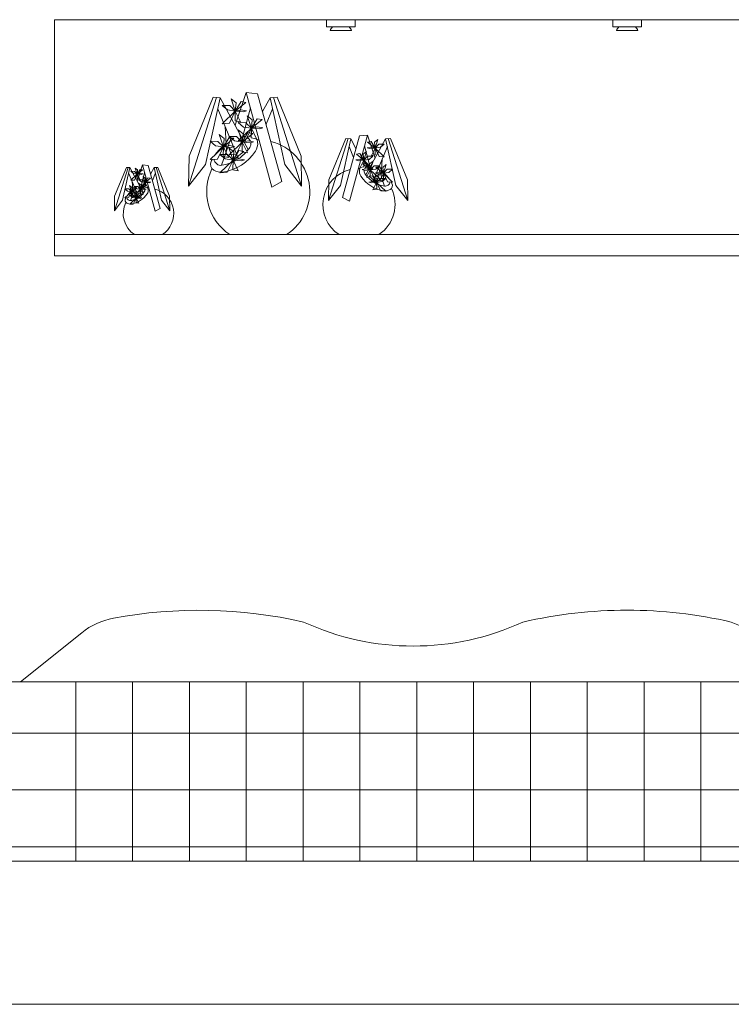
# Model space of a CAD drawing. Units: inches. Extents: x 1994 to 3075, y 3517 to 3950.
# Tile 27 of 58: x 1994.49073 to 1994.52987, y 3553.60329 to 3553.6574. Entities that reach past the tile are written whole.
import ezdxf

# ---------------------------------------------------------------- set-up
doc = ezdxf.new("R2010")
doc.units = ezdxf.units.IN
doc.layers.add('A-FURN-REFR', color=8, linetype='Continuous', lineweight=13)

msp = doc.modelspace()

# ---------------------------------------------------------------- linework, layer by layer
at = {"layer": 'A-FURN-REFR'}
for p, q in [((1994.492639873162, 3553.657398571457), (1994.555631999147, 3553.657398571457)), ((1994.492639873162, 3553.657398571457), (1994.492639873162, 3553.644427213402)), ((1994.507600503083, 3553.657004870669), (1994.507600503083, 3553.657398571457)), ((1994.507600503083, 3553.657398571457), (1994.509175306233, 3553.657398571457)), ((1994.509175306233, 3553.657004870669), (1994.509175306233, 3553.657398571457)), ((1994.52334853458, 3553.657004870669), (1994.52334853458, 3553.657398571457)), ((1994.52334853458, 3553.657398571457), (1994.524923337729, 3553.657398571457)), ((1994.524923337729, 3553.657004870669), (1994.524923337729, 3553.657398571457)), ((1994.507600503083, 3553.657004870669), (1994.509175306233, 3553.657004870669)), ((1994.507797353477, 3553.656808020276), (1994.50897845584, 3553.656808020276)), ((1994.523348534579, 3553.657004870669), (1994.524923337729, 3553.657004870669)), ((1994.523545384973, 3553.656808020276), (1994.524726487336, 3553.656808020276)), ((1994.502576726892, 3553.651601865461), (1994.503185007687, 3553.653402428091)), ((1994.504591077029, 3553.648203264901), (1994.503185007687, 3553.653402428091)), ((1994.503185007687, 3553.653402428091), (1994.503814087741, 3553.653332248833)), ((1994.503814087741, 3553.653332248833), (1994.505147097463, 3553.648511813597)), ((1994.501557670898, 3553.653122215547), (1994.500019605817, 3553.648259076231)), ((1994.500042747255, 3553.649899375615), (1994.501361075979, 3553.653133767314)), ((1994.501754265817, 3553.653110663779), (1994.500940059187, 3553.649441019369)), ((1994.501361075979, 3553.653133767314), (1994.501754265817, 3553.653110663779)), ((1994.503302966856, 3553.650269584008), (1994.501754265817, 3553.653110663779)), ((1994.502586648582, 3553.652376770545), (1994.502357374983, 3553.653055718957)), ((1994.502357374983, 3553.653055718957), (1994.502632143048, 3553.652839128945)), ((1994.502586648582, 3553.652376770545), (1994.502901656143, 3553.652903470256)), ((1994.503168087577, 3553.652856889033), (1994.502586648582, 3553.652376770545)), ((1994.502632143048, 3553.652839128945), (1994.502586648582, 3553.652376770545)), ((1994.502901656143, 3553.652903470256), (1994.503168087577, 3553.652856889033)), ((1994.504084833384, 3553.652353177328), (1994.504497746835, 3553.653110663779)), ((1994.504890936673, 3553.653133767314), (1994.504497746835, 3553.653110663779)), ((1994.504497746835, 3553.653110663779), (1994.505311953465, 3553.649441019369)), ((1994.504694341754, 3553.653122215547), (1994.506232406834, 3553.648259076231)), ((1994.506209265397, 3553.649899375615), (1994.504890936673, 3553.653133767314)), ((1994.501620007458, 3553.65250555886), (1994.502755091202, 3553.649751667343)), ((1994.501862205752, 3553.651685138613), (1994.502586648582, 3553.652376770545)), ((1994.502281794018, 3553.652685614927), (1994.501864021999, 3553.652690691328)), ((1994.501864021999, 3553.652690691328), (1994.502157458303, 3553.652440933305)), ((1994.502157458303, 3553.652440933305), (1994.502586648582, 3553.652376770545)), ((1994.502586648582, 3553.652376770545), (1994.502261309524, 3553.65171323023)), ((1994.502586648582, 3553.652376770545), (1994.502281794018, 3553.652685614927)), ((1994.502586648582, 3553.652376770545), (1994.502578490516, 3553.651848076031)), ((1994.502586648582, 3553.652376770545), (1994.502915247888, 3553.652452530144)), ((1994.502870840114, 3553.651794244866), (1994.502586648582, 3553.652376770545)), ((1994.503023088817, 3553.652338526031), (1994.502586648582, 3553.652376770545)), ((1994.502915247888, 3553.652452530144), (1994.50320759741, 3553.652398698999)), ((1994.502970969925, 3553.650878629744), (1994.503416085914, 3553.652547979897)), ((1994.50320759741, 3553.652398698999), (1994.503023088817, 3553.652338526031)), ((1994.504632005194, 3553.65250555886), (1994.504279317495, 3553.651649883085)), ((1994.502261309524, 3553.65171323023), (1994.501862205752, 3553.651685138613)), ((1994.502578490516, 3553.651848076031), (1994.502870840114, 3553.651794244866)), ((1994.503169538199, 3553.651739866096), (1994.50275176618, 3553.651744942497)), ((1994.50275176618, 3553.651744942497), (1994.503045202485, 3553.651495184475)), ((1994.503474392764, 3553.651431021715), (1994.503169538199, 3553.651739866096)), ((1994.503474392764, 3553.651431021715), (1994.503245119164, 3553.652109970126)), ((1994.503245119164, 3553.652109970126), (1994.50351988723, 3553.651893380115)), ((1994.503474392764, 3553.651431021715), (1994.503789400325, 3553.651957721426)), ((1994.504055831759, 3553.651911140202), (1994.503474392764, 3553.651431021715)), ((1994.50351988723, 3553.651893380115), (1994.503474392764, 3553.651431021715)), ((1994.503789400325, 3553.651957721426), (1994.504055831759, 3553.651911140202)), ((1994.502021550454, 3553.651531352458), (1994.502109068058, 3553.650217555736)), ((1994.502965155948, 3553.650673222332), (1994.502735882347, 3553.651352170744)), ((1994.502735882347, 3553.651352170744), (1994.503010650413, 3553.651135580733)), ((1994.502749949934, 3553.650739389782), (1994.503474392764, 3553.651431021715)), ((1994.502965155948, 3553.650673222332), (1994.503280163509, 3553.651199922044)), ((1994.503045202485, 3553.651495184475), (1994.503474392764, 3553.651431021715)), ((1994.503474392764, 3553.651431021715), (1994.503149053706, 3553.6507674814)), ((1994.503280163509, 3553.651199922044), (1994.503546594942, 3553.65115334082)), ((1994.503474392764, 3553.651431021715), (1994.503466234698, 3553.650902327201)), ((1994.503474392764, 3553.651431021715), (1994.503802992069, 3553.651506781313)), ((1994.503758584295, 3553.650848496036), (1994.503474392764, 3553.651431021715)), ((1994.503910832998, 3553.651392777201), (1994.503474392764, 3553.651431021715)), ((1994.503802992069, 3553.651506781313), (1994.504095341592, 3553.651452950168)), ((1994.504095341592, 3553.651452950168), (1994.503910832998, 3553.651392777201)), ((1994.501625482097, 3553.650714359771), (1994.501207710078, 3553.650719436171)), ((1994.501207710078, 3553.650719436171), (1994.501501146383, 3553.650469678149)), ((1994.501930336662, 3553.650405515389), (1994.501625482097, 3553.650714359771)), ((1994.501930336662, 3553.650405515389), (1994.501701063062, 3553.651084463801)), ((1994.501701063062, 3553.651084463801), (1994.501975831128, 3553.65086787379)), ((1994.501831630469, 3553.649396316995), (1994.502313564127, 3553.650822881405)), ((1994.501930336662, 3553.650405515389), (1994.502245344223, 3553.6509322151)), ((1994.502511775657, 3553.650885633877), (1994.501930336662, 3553.650405515389)), ((1994.501975831128, 3553.65086787379), (1994.501930336662, 3553.650405515389)), ((1994.502240713117, 3553.6499815904), (1994.502965155948, 3553.650673222332)), ((1994.502660301383, 3553.650982066714), (1994.502242529364, 3553.650987143115)), ((1994.502242529364, 3553.650987143115), (1994.502535965668, 3553.650737385092)), ((1994.502245344223, 3553.6509322151), (1994.502511775657, 3553.650885633877)), ((1994.502535965668, 3553.650737385092), (1994.502965155948, 3553.650673222332)), ((1994.502965155948, 3553.650673222332), (1994.502639816889, 3553.650009682018)), ((1994.502965155948, 3553.650673222332), (1994.502660301383, 3553.650982066714)), ((1994.503149053706, 3553.6507674814), (1994.502749949934, 3553.650739389782)), ((1994.502965155948, 3553.650673222332), (1994.502956997882, 3553.650144527818)), ((1994.503546594942, 3553.65115334082), (1994.502965155948, 3553.650673222332)), ((1994.503010650413, 3553.651135580733), (1994.502965155948, 3553.650673222332)), ((1994.502965155948, 3553.650673222332), (1994.503293755253, 3553.650748981931)), ((1994.503249347479, 3553.650090696653), (1994.502965155948, 3553.650673222332)), ((1994.503401596182, 3553.650634977819), (1994.502965155948, 3553.650673222332)), ((1994.503293755253, 3553.650748981931), (1994.503586104775, 3553.650695150787)), ((1994.503586104775, 3553.650695150787), (1994.503401596182, 3553.650634977819)), ((1994.503466234698, 3553.650902327201), (1994.503758584295, 3553.650848496036)), ((1994.508796361508, 3553.650861815234), (1994.507719715952, 3553.647457617712)), ((1994.507735914958, 3553.648605827281), (1994.508658745065, 3553.65086990147)), ((1994.508933977952, 3553.650853728996), (1994.508364033311, 3553.648284977909)), ((1994.509412539317, 3553.651008838534), (1994.508479432512, 3553.647634533869)), ((1994.508658745065, 3553.65086990147), (1994.508933977952, 3553.650853728996)), ((1994.508868646816, 3553.64741854978), (1994.509852895355, 3553.651057964014)), ((1994.509223017368, 3553.65032348848), (1994.508933977952, 3553.650853728996)), ((1994.509852895355, 3553.651057964014), (1994.509412539317, 3553.651008838534)), ((1994.509770323937, 3553.648864973156), (1994.510854414664, 3553.650853728996)), ((1994.510278691912, 3553.649797570173), (1994.509852895355, 3553.651057964014)), ((1994.510051241436, 3553.65070869353), (1994.509864739432, 3553.650676086674)), ((1994.509864739432, 3553.650676086674), (1994.510271746728, 3553.650340003732)), ((1994.510271746728, 3553.650340003732), (1994.510051241436, 3553.65070869353)), ((1994.510432238248, 3553.650815267621), (1994.510239900602, 3553.650663654612)), ((1994.510239900602, 3553.650663654612), (1994.510271746728, 3553.650340003732)), ((1994.510271746728, 3553.650340003732), (1994.510432238248, 3553.650815267621)), ((1994.511129647551, 3553.65086990147), (1994.510854414664, 3553.650853728996)), ((1994.510854414664, 3553.650853728996), (1994.511424359305, 3553.648284977909)), ((1994.510992031107, 3553.650861815234), (1994.512068676664, 3553.647457617712)), ((1994.512052477658, 3553.648605827281), (1994.511129647551, 3553.65086990147)), ((1994.501205893832, 3553.649713883457), (1994.501930336662, 3553.650405515389)), ((1994.501501146383, 3553.650469678149), (1994.501930336662, 3553.650405515389)), ((1994.501930336662, 3553.650405515389), (1994.501604997604, 3553.649741975074)), ((1994.501930336662, 3553.650405515389), (1994.501922178596, 3553.649876820875)), ((1994.501930336662, 3553.650405515389), (1994.502258935968, 3553.650481274987)), ((1994.502214528194, 3553.64982298971), (1994.501930336662, 3553.650405515389)), ((1994.502366776896, 3553.650367270876), (1994.501930336662, 3553.650405515389)), ((1994.50246636318, 3553.649684181244), (1994.50223708958, 3553.650363129655)), ((1994.50223708958, 3553.650363129655), (1994.502511857646, 3553.650146539644)), ((1994.502258935968, 3553.650481274987), (1994.50255128549, 3553.650427443843)), ((1994.50255128549, 3553.650427443843), (1994.502366776896, 3553.650367270876)), ((1994.50246636318, 3553.649684181244), (1994.502781370741, 3553.650210880955)), ((1994.503047802175, 3553.650164299731), (1994.50246636318, 3553.649684181244)), ((1994.502511857646, 3553.650146539644), (1994.50246636318, 3553.649684181244)), ((1994.502781370741, 3553.650210880955), (1994.503047802175, 3553.650164299731)), ((1994.502956997882, 3553.650144527818), (1994.503249347479, 3553.650090696653)), ((1994.5088399971, 3553.650430155552), (1994.509086878489, 3553.64983118251)), ((1994.509810817321, 3553.650153243439), (1994.509618479676, 3553.650001630431)), ((1994.509650325801, 3553.649677979551), (1994.509810817321, 3553.650153243439)), ((1994.510002721789, 3553.649291305171), (1994.509691140596, 3553.650459850279)), ((1994.510041727215, 3553.650393035451), (1994.509837082549, 3553.65035535365)), ((1994.509837082549, 3553.65035535365), (1994.509966238565, 3553.650313232573)), ((1994.509966238565, 3553.650313232573), (1994.510271746728, 3553.650340003732)), ((1994.510271746728, 3553.650340003732), (1994.510041727215, 3553.650393035451)), ((1994.510072812656, 3553.649932235757), (1994.510271746728, 3553.650340003732)), ((1994.510948395516, 3553.650430155552), (1994.510153836895, 3553.648502431491)), ((1994.510271746728, 3553.650340003732), (1994.510485144924, 3553.650556194799)), ((1994.510572179924, 3553.650384917664), (1994.510271746728, 3553.650340003732)), ((1994.510271746728, 3553.650340003732), (1994.510499484069, 3553.649875525512)), ((1994.51077885671, 3553.64985586138), (1994.510271746728, 3553.650340003732)), ((1994.510271746728, 3553.650340003732), (1994.510277457374, 3553.649969917572)), ((1994.510485144924, 3553.650556194799), (1994.510777585337, 3553.650559748279)), ((1994.510777585337, 3553.650559748279), (1994.510572179924, 3553.650384917664)), ((1994.500019605817, 3553.648259076231), (1994.500042747255, 3553.649899375615)), ((1994.501604997604, 3553.649741975074), (1994.501205893832, 3553.649713883457)), ((1994.50174192035, 3553.648992549311), (1994.50246636318, 3553.649684181244)), ((1994.502161508616, 3553.649993025626), (1994.501743736596, 3553.649998102026)), ((1994.501743736596, 3553.649998102026), (1994.502037172901, 3553.649748344003)), ((1994.501922178596, 3553.649876820875), (1994.502214528194, 3553.64982298971)), ((1994.502037172901, 3553.649748344003), (1994.50246636318, 3553.649684181244)), ((1994.50246636318, 3553.649684181244), (1994.502141024122, 3553.649020640929)), ((1994.50246636318, 3553.649684181244), (1994.502161508616, 3553.649993025626)), ((1994.502639816889, 3553.650009682018), (1994.502240713117, 3553.6499815904)), ((1994.50246636318, 3553.649684181244), (1994.502458205115, 3553.64915548673)), ((1994.50246636318, 3553.649684181244), (1994.502794962486, 3553.649759940842)), ((1994.502750554712, 3553.649101655564), (1994.50246636318, 3553.649684181244)), ((1994.502902803414, 3553.649645936729), (1994.50246636318, 3553.649684181244)), ((1994.502664672884, 3553.649729902166), (1994.502703713299, 3553.64987631821)), ((1994.502794962486, 3553.649759940842), (1994.503087312008, 3553.649706109697)), ((1994.503087312008, 3553.649706109697), (1994.502902803414, 3553.649645936729)), ((1994.506232406834, 3553.648259076231), (1994.506209265397, 3553.649899375615)), ((1994.509420306287, 3553.649731011269), (1994.509215661622, 3553.649693329469)), ((1994.509215661622, 3553.649693329469), (1994.509344817637, 3553.649651208391)), ((1994.509429820509, 3553.650046669349), (1994.509243318505, 3553.650014062492)), ((1994.509243318505, 3553.650014062492), (1994.509650325801, 3553.649677979551)), ((1994.509344817637, 3553.649651208391), (1994.509650325801, 3553.649677979551)), ((1994.509650325801, 3553.649677979551), (1994.509420306287, 3553.649731011269)), ((1994.509650325801, 3553.649677979551), (1994.509429820509, 3553.650046669349)), ((1994.509451391729, 3553.649270211575), (1994.509650325801, 3553.649677979551)), ((1994.509618479676, 3553.650001630431), (1994.509650325801, 3553.649677979551)), ((1994.509650325801, 3553.649677979551), (1994.509863723996, 3553.649894170618)), ((1994.509950758996, 3553.649722893482), (1994.509650325801, 3553.649677979551)), ((1994.509650325801, 3553.649677979551), (1994.509878063142, 3553.64921350133)), ((1994.510157435783, 3553.649193837198), (1994.509650325801, 3553.649677979551)), ((1994.509650325801, 3553.649677979551), (1994.509656036447, 3553.649307893391)), ((1994.509863723996, 3553.649894170618), (1994.51015616441, 3553.649897724098)), ((1994.51015616441, 3553.649897724098), (1994.509950758996, 3553.649722893482)), ((1994.510167283093, 3553.649622783872), (1994.509974945447, 3553.649471170864)), ((1994.510006791573, 3553.649147519983), (1994.510167283093, 3553.649622783872)), ((1994.510277457374, 3553.649969917572), (1994.510072812656, 3553.649932235757)), ((1994.510499484069, 3553.649875525512), (1994.51077885671, 3553.64985586138)), ((1994.510667315418, 3553.649748211071), (1994.510606053095, 3553.648828553366)), ((1994.496690646978, 3553.649279535251), (1994.495936995089, 3553.646896596986)), ((1994.495948334393, 3553.647700343685), (1994.496594315467, 3553.649285195616)), ((1994.496786978488, 3553.649273874884), (1994.49638801724, 3553.647475749123)), ((1994.496594315467, 3553.649285195616), (1994.496786978488, 3553.649273874884)), ((1994.497545841997, 3553.647881745797), (1994.496786978488, 3553.649273874884)), ((1994.497045467307, 3553.649065600947), (1994.496840759017, 3553.649068088383)), ((1994.496840759017, 3553.649068088383), (1994.496984542807, 3553.648945706952)), ((1994.497194846043, 3553.6489142672), (1994.497045467307, 3553.649065600947)), ((1994.497194846043, 3553.6489142672), (1994.497082501979, 3553.649246951922)), ((1994.497082501979, 3553.649246951922), (1994.497217138331, 3553.649140822816)), ((1994.497189984415, 3553.648534563708), (1994.497488042005, 3553.649416839397)), ((1994.497194846043, 3553.6489142672), (1994.497349199749, 3553.649172350058)), ((1994.497479751151, 3553.649149525259), (1994.497194846043, 3553.6489142672)), ((1994.497217138331, 3553.649140822816), (1994.497194846043, 3553.6489142672)), ((1994.497349199749, 3553.649172350058), (1994.497479751151, 3553.649149525259)), ((1994.498177015982, 3553.646869249434), (1994.497488042005, 3553.649416839397)), ((1994.497488042005, 3553.649416839397), (1994.497796291232, 3553.649382451561)), ((1994.497796291232, 3553.649382451561), (1994.498449465995, 3553.647020438296)), ((1994.497928956596, 3553.648902706524), (1994.498131284187, 3553.649273874884)), ((1994.498323947208, 3553.649285195616), (1994.498131284187, 3553.649273874884)), ((1994.498131284187, 3553.649273874884), (1994.498530245436, 3553.647475749123)), ((1994.498227615698, 3553.649279535251), (1994.498981267587, 3553.646896596986)), ((1994.498969928282, 3553.647700343685), (1994.498323947208, 3553.649285195616)), ((1994.500940059187, 3553.649441019369), (1994.500019605817, 3553.648259076231)), ((1994.502141024122, 3553.649020640929), (1994.50174192035, 3553.648992549311)), ((1994.502458205115, 3553.64915548673), (1994.502750554712, 3553.649101655564)), ((1994.505311953465, 3553.649441019369), (1994.506232406834, 3553.648259076231)), ((1994.509656036447, 3553.649307893391), (1994.509451391729, 3553.649270211575)), ((1994.509776772059, 3553.649200551702), (1994.509572127393, 3553.649162869901)), ((1994.509572127393, 3553.649162869901), (1994.509701283409, 3553.649120748823)), ((1994.50978628628, 3553.649516209781), (1994.509599784277, 3553.649483602924)), ((1994.509599784277, 3553.649483602924), (1994.510006791573, 3553.649147519983)), ((1994.509701283409, 3553.649120748823), (1994.510006791573, 3553.649147519983)), ((1994.510006791573, 3553.649147519983), (1994.509776772059, 3553.649200551702)), ((1994.510006791573, 3553.649147519983), (1994.50978628628, 3553.649516209781)), ((1994.5098078575, 3553.648739752008), (1994.510006791573, 3553.649147519983)), ((1994.509878063142, 3553.64921350133), (1994.510157435783, 3553.649193837198)), ((1994.509974945447, 3553.649471170864), (1994.510006791573, 3553.649147519983)), ((1994.510006791573, 3553.649147519983), (1994.510220189768, 3553.649363711051)), ((1994.510307224768, 3553.649192433915), (1994.510006791573, 3553.649147519983)), ((1994.510006791573, 3553.649147519983), (1994.510234528913, 3553.648683041763)), ((1994.510513901554, 3553.648663377631), (1994.510006791573, 3553.649147519983)), ((1994.510006791573, 3553.649147519983), (1994.510012502219, 3553.648777433823)), ((1994.510220189768, 3553.649363711051), (1994.510512630181, 3553.649367264531)), ((1994.510501145559, 3553.649013156841), (1994.510296500893, 3553.648975475041)), ((1994.510512630181, 3553.649367264531), (1994.510307224768, 3553.649192433915)), ((1994.51051065978, 3553.64932881492), (1994.510324157776, 3553.649296208064)), ((1994.510324157776, 3553.649296208064), (1994.510731165073, 3553.648960125123)), ((1994.510800259408, 3553.648253686247), (1994.510462905848, 3553.649252281334)), ((1994.510731165073, 3553.648960125123), (1994.510501145559, 3553.649013156841)), ((1994.510731165073, 3553.648960125123), (1994.51051065978, 3553.64932881492)), ((1994.510891656593, 3553.649435389012), (1994.510699318947, 3553.649283776003)), ((1994.510699318947, 3553.649283776003), (1994.510731165073, 3553.648960125123)), ((1994.510731165073, 3553.648960125123), (1994.510891656593, 3553.649435389012)), ((1994.510731165073, 3553.648960125123), (1994.510944563268, 3553.64917631619)), ((1994.511031598268, 3553.649005039055), (1994.510731165073, 3553.648960125123)), ((1994.510944563268, 3553.64917631619), (1994.511237003681, 3553.64917986967)), ((1994.511237003681, 3553.64917986967), (1994.511031598268, 3553.649005039055)), ((1994.496721191893, 3553.648977373474), (1994.497277382927, 3553.647627966631)), ((1994.496839869056, 3553.648575367553), (1994.497194846043, 3553.6489142672)), ((1994.497035429905, 3553.648589132445), (1994.496839869056, 3553.648575367553)), ((1994.496917947961, 3553.648500012338), (1994.496960831586, 3553.647856251944)), ((1994.496984542807, 3553.648945706952), (1994.497194846043, 3553.6489142672)), ((1994.497194846043, 3553.6489142672), (1994.497035429905, 3553.648589132445)), ((1994.497194846043, 3553.6489142672), (1994.497190848591, 3553.648655206888)), ((1994.497190848591, 3553.648655206888), (1994.497334099894, 3553.648628829617)), ((1994.497194846043, 3553.6489142672), (1994.497355859703, 3553.648951389404)), ((1994.497334099894, 3553.648628829617), (1994.497194846043, 3553.6489142672)), ((1994.497408701758, 3553.648895527388), (1994.497194846043, 3553.6489142672)), ((1994.497480461956, 3553.648602184021), (1994.497275753667, 3553.648604671457)), ((1994.497275753667, 3553.648604671457), (1994.497419537455, 3553.648482290026)), ((1994.497355859703, 3553.648951389404), (1994.497499110969, 3553.648925012142)), ((1994.497383163501, 3553.648180178207), (1994.497601270336, 3553.648998159783)), ((1994.497499110969, 3553.648925012142), (1994.497408701758, 3553.648895527388)), ((1994.497419537455, 3553.648482290026), (1994.497629840692, 3553.648450850273)), ((1994.497629840692, 3553.648450850273), (1994.497480461956, 3553.648602184021)), ((1994.497629840692, 3553.648450850273), (1994.497517496628, 3553.648783534995)), ((1994.497517496628, 3553.648783534995), (1994.497652132981, 3553.648677405889)), ((1994.497629840692, 3553.648450850273), (1994.497784194398, 3553.648708933132)), ((1994.4979147458, 3553.648686108332), (1994.497629840692, 3553.648450850273)), ((1994.497652132981, 3553.648677405889), (1994.497629840692, 3553.648450850273)), ((1994.497629840692, 3553.648450850273), (1994.497790854352, 3553.648487972476)), ((1994.497784194398, 3553.648708933132), (1994.4979147458, 3553.648686108332)), ((1994.497790854352, 3553.648487972476), (1994.497934105618, 3553.648461595216)), ((1994.497934105618, 3553.648461595216), (1994.497843696407, 3553.648432110462)), ((1994.498197070783, 3553.648977373474), (1994.498024253811, 3553.648558092345)), ((1994.505147097463, 3553.648511813597), (1994.504591077029, 3553.648203264901)), ((1994.507719715952, 3553.647457617712), (1994.507735914958, 3553.648605827281)), ((1994.510012502219, 3553.648777433823), (1994.5098078575, 3553.648739752008)), ((1994.510125926996, 3553.64850822294), (1994.509921282331, 3553.648470541139)), ((1994.509921282331, 3553.648470541139), (1994.510050438346, 3553.648428420061)), ((1994.510135441217, 3553.648823881019), (1994.509948939214, 3553.648791274162)), ((1994.509948939214, 3553.648791274162), (1994.51035594651, 3553.648455191221)), ((1994.51035594651, 3553.648455191221), (1994.510125926996, 3553.64850822294)), ((1994.51035594651, 3553.648455191221), (1994.510135441217, 3553.648823881019)), ((1994.510217129717, 3553.648487195867), (1994.510189801427, 3553.648589687097)), ((1994.510234528913, 3553.648683041763), (1994.510513901554, 3553.648663377631)), ((1994.510296500893, 3553.648975475041), (1994.510425656909, 3553.648933353963)), ((1994.51051643803, 3553.648930455109), (1994.510324100384, 3553.648778842101)), ((1994.510324100384, 3553.648778842101), (1994.51035594651, 3553.648455191221)), ((1994.51035594651, 3553.648455191221), (1994.51051643803, 3553.648930455109)), ((1994.51035594651, 3553.648455191221), (1994.510569344705, 3553.648671382288)), ((1994.510656379705, 3553.648500105153), (1994.51035594651, 3553.648455191221)), ((1994.510425656909, 3553.648933353963), (1994.510731165073, 3553.648960125123)), ((1994.510532231, 3553.648552357147), (1994.510731165073, 3553.648960125123)), ((1994.510736875719, 3553.648590038963), (1994.510532231, 3553.648552357147)), ((1994.510569344705, 3553.648671382288), (1994.510861785119, 3553.648674935768)), ((1994.510861785119, 3553.648674935768), (1994.510656379705, 3553.648500105153)), ((1994.510731165073, 3553.648960125123), (1994.510958902413, 3553.648495646902)), ((1994.511238275054, 3553.64847598277), (1994.510731165073, 3553.648960125123)), ((1994.510731165073, 3553.648960125123), (1994.510736875719, 3553.648590038963)), ((1994.510958902413, 3553.648495646902), (1994.511238275054, 3553.64847598277)), ((1994.512068676664, 3553.647457617712), (1994.512052477658, 3553.648605827281)), ((1994.496518276216, 3553.647609452526), (1994.496873253202, 3553.647948352174)), ((1994.496723874466, 3553.648099685921), (1994.496519166176, 3553.648102173357)), ((1994.496519166176, 3553.648102173357), (1994.496662949966, 3553.647979791926)), ((1994.496662949966, 3553.647979791926), (1994.496873253202, 3553.647948352174)), ((1994.496873253202, 3553.647948352174), (1994.496713837064, 3553.64762321742)), ((1994.496873253202, 3553.647948352174), (1994.496723874466, 3553.648099685921)), ((1994.496873253202, 3553.647948352174), (1994.496760909138, 3553.648281036895)), ((1994.496760909138, 3553.648281036895), (1994.496895545491, 3553.648174907789)), ((1994.496824887168, 3553.64745384496), (1994.49706103466, 3553.648152861522)), ((1994.496873253202, 3553.647948352174), (1994.49686925575, 3553.647689291862)), ((1994.496873253202, 3553.647948352174), (1994.497027606907, 3553.648206435032)), ((1994.49715815831, 3553.648183610232), (1994.496873253202, 3553.647948352174)), ((1994.496895545491, 3553.648174907789), (1994.496873253202, 3553.647948352174)), ((1994.496873253202, 3553.647948352174), (1994.497034266862, 3553.647985474376)), ((1994.497012507053, 3553.64766291459), (1994.496873253202, 3553.647948352174)), ((1994.497087108917, 3553.647929612362), (1994.496873253202, 3553.647948352174)), ((1994.497135906196, 3553.647594898443), (1994.497023562132, 3553.647927583164)), ((1994.497023562132, 3553.647927583164), (1994.497158198484, 3553.647821454058)), ((1994.497025337665, 3553.647740628929), (1994.497380314652, 3553.648079528576)), ((1994.497230935916, 3553.648230862323), (1994.497026227626, 3553.648233349759)), ((1994.497026227626, 3553.648233349759), (1994.497170011416, 3553.648110968328)), ((1994.497027606907, 3553.648206435032), (1994.49715815831, 3553.648183610232)), ((1994.497034266862, 3553.647985474376), (1994.497177518128, 3553.647959097116)), ((1994.497177518128, 3553.647959097116), (1994.497087108917, 3553.647929612362)), ((1994.497170011416, 3553.648110968328), (1994.497380314652, 3553.648079528576)), ((1994.497380314652, 3553.648079528576), (1994.497220898514, 3553.647754393821)), ((1994.497380314652, 3553.648079528576), (1994.497230935916, 3553.648230862323)), ((1994.497380314652, 3553.648079528576), (1994.497267970588, 3553.648412213298)), ((1994.497267970588, 3553.648412213298), (1994.497402606941, 3553.648306084192)), ((1994.497274863705, 3553.648111950626), (1994.497629840692, 3553.648450850273)), ((1994.497470424554, 3553.648125715518), (1994.497274863705, 3553.648111950626)), ((1994.497380314652, 3553.648079528576), (1994.4973763172, 3553.647820468264)), ((1994.497380314652, 3553.648079528576), (1994.497534668357, 3553.648337611434)), ((1994.49766521976, 3553.648314786635), (1994.497380314652, 3553.648079528576)), ((1994.497402606941, 3553.648306084192), (1994.497380314652, 3553.648079528576)), ((1994.497380314652, 3553.648079528576), (1994.497541328312, 3553.648116650779)), ((1994.497519568503, 3553.647794090993), (1994.497380314652, 3553.648079528576)), ((1994.497594170367, 3553.648060788764), (1994.497380314652, 3553.648079528576)), ((1994.497629840692, 3553.648450850273), (1994.497470424554, 3553.648125715518)), ((1994.497534668357, 3553.648337611434), (1994.49766521976, 3553.648314786635)), ((1994.497541328312, 3553.648116650779), (1994.497684579578, 3553.648090273518)), ((1994.497684579578, 3553.648090273518), (1994.497594170367, 3553.648060788764)), ((1994.497629840692, 3553.648450850273), (1994.49762584324, 3553.648191789961)), ((1994.49762584324, 3553.648191789961), (1994.497769094543, 3553.648165412691)), ((1994.497769094543, 3553.648165412691), (1994.497629840692, 3553.648450850273)), ((1994.497843696407, 3553.648432110462), (1994.497629840692, 3553.648450850273)), ((1994.508364033311, 3553.648284977909), (1994.507719715952, 3553.647457617712)), ((1994.510050438346, 3553.648428420061), (1994.51035594651, 3553.648455191221)), ((1994.510157012438, 3553.648047423246), (1994.51035594651, 3553.648455191221)), ((1994.510361657156, 3553.648085105062), (1994.510157012438, 3553.648047423246)), ((1994.51035594651, 3553.648455191221), (1994.510583683851, 3553.647990713)), ((1994.510863056491, 3553.647971048869), (1994.51035594651, 3553.648455191221)), ((1994.51035594651, 3553.648455191221), (1994.510361657156, 3553.648085105062)), ((1994.510583683851, 3553.647990713), (1994.510863056491, 3553.647971048869)), ((1994.511424359305, 3553.648284977909), (1994.512068676664, 3553.647457617712)), ((1994.495936995089, 3553.646896596986), (1994.495948334393, 3553.647700343685)), ((1994.49638801724, 3553.647475749123), (1994.495936995089, 3553.646896596986)), ((1994.496713837064, 3553.64762321742), (1994.496518276216, 3553.647609452526)), ((1994.496780929209, 3553.647255998795), (1994.497135906196, 3553.647594898443)), ((1994.49698652746, 3553.647746232189), (1994.496781819171, 3553.647748719625)), ((1994.496781819171, 3553.647748719625), (1994.49692560296, 3553.647626338194)), ((1994.49686925575, 3553.647689291862), (1994.497012507053, 3553.64766291459)), ((1994.49692560296, 3553.647626338194), (1994.497135906196, 3553.647594898443)), ((1994.497135906196, 3553.647594898443), (1994.496976490058, 3553.647269763688)), ((1994.497135906196, 3553.647594898443), (1994.49698652746, 3553.647746232189)), ((1994.497220898514, 3553.647754393821), (1994.497025337665, 3553.647740628929)), ((1994.497135906196, 3553.647594898443), (1994.497131908744, 3553.647335838131)), ((1994.497135906196, 3553.647594898443), (1994.497290259901, 3553.6478529813)), ((1994.497420811304, 3553.647830156501), (1994.497135906196, 3553.647594898443)), ((1994.497158198484, 3553.647821454058), (1994.497135906196, 3553.647594898443)), ((1994.497135906196, 3553.647594898443), (1994.497296919856, 3553.647632020645)), ((1994.497275160047, 3553.647309460859), (1994.497135906196, 3553.647594898443)), ((1994.497349761911, 3553.64757615863), (1994.497135906196, 3553.647594898443)), ((1994.497233077951, 3553.647617301694), (1994.497252207754, 3553.647689045555)), ((1994.497290259901, 3553.6478529813), (1994.497420811304, 3553.647830156501)), ((1994.497296919856, 3553.647632020645), (1994.497440171122, 3553.647605643385)), ((1994.497440171122, 3553.647605643385), (1994.497349761911, 3553.64757615863)), ((1994.4973763172, 3553.647820468264), (1994.497519568503, 3553.647794090993)), ((1994.498530245436, 3553.647475749123), (1994.498981267587, 3553.646896596986)), ((1994.498981267587, 3553.646896596986), (1994.498969928282, 3553.647700343685)), ((1994.508479432512, 3553.647634533869), (1994.508868646816, 3553.64741854978)), ((1994.496976490058, 3553.647269763688), (1994.496780929209, 3553.647255998795)), ((1994.497131908744, 3553.647335838131), (1994.497275160047, 3553.647309460859)), ((1994.498449465995, 3553.647020438296), (1994.498177015982, 3553.646869249434)), ((1994.492639873162, 3553.645587547835), (1994.555631999147, 3553.645587547835)), ((1994.492639873162, 3553.644427213402), (1994.555631999146, 3553.644427213402)), ((1994.490767123576, 3553.621010566067), (1994.494145291931, 3553.623713100752)), ((1994.485750109383, 3553.621010566067), (1994.562521762926, 3553.621010566067)), ((1994.490767123576, 3553.621010566067), (1994.490767123576, 3553.621010566067)), ((1994.493814222183, 3553.611168046383), (1994.493814222183, 3553.621010566067)), ((1994.496939222183, 3553.611168046383), (1994.496939222183, 3553.621010566067)), ((1994.500064222183, 3553.611168046383), (1994.500064222183, 3553.621010566067)), ((1994.503189222183, 3553.611168046383), (1994.503189222183, 3553.621010566067)), ((1994.506314222183, 3553.611168046383), (1994.506314222183, 3553.621010566067)), ((1994.509439222183, 3553.611168046383), (1994.509439222183, 3553.621010566067)), ((1994.512564222183, 3553.611168046383), (1994.512564222183, 3553.621010566067)), ((1994.515689222183, 3553.611168046383), (1994.515689222183, 3553.621010566067)), ((1994.518814222183, 3553.611168046383), (1994.518814222183, 3553.621010566067)), ((1994.521939222183, 3553.611168046383), (1994.521939222183, 3553.621010566067)), ((1994.525064222183, 3553.611168046383), (1994.525064222183, 3553.621010566067)), ((1994.528189222183, 3553.611168046383), (1994.528189222183, 3553.621010566067)), ((1994.483781605446, 3553.618198825726), (1994.564490266863, 3553.618198825726)), ((1994.483781605446, 3553.615073825726), (1994.564490266863, 3553.615073825726)), ((1994.483781633293, 3553.611948825726), (1994.564490239016, 3553.611948825726)), ((1994.48456900702, 3553.611168046383), (1994.563702865288, 3553.611168046383)), ((1994.602439621408, 3553.603294030634), (1994.442865031001, 3553.603294030634))]:
    msp.add_line(p, q, dxfattribs=at)
for centre, radius, start, end in [((1994.508387904658, 3553.656561957283), 0.0006397637796166, 136.1869385529525, 157.3801350610466), ((1994.508387904658, 3553.656561957283), 0.0006397637796166, 22.61986494091335, 43.81306144798317), ((1994.524135936154, 3553.656561957283), 0.0006397637796166, 136.1869385529525, 157.3801350610466), ((1994.524135936154, 3553.656561957283), 0.0006397637796166, 22.61986494091335, 43.81306144798317), ((1994.503470773054, 3553.648547092116), 0.0024566929133858, 97.49545616133652, 101.2899186130162), ((1994.503063810613, 3553.650585606823), 0.0003779527559055, 79.17721224419212, 101.2899186126917), ((1994.503063810613, 3553.650585606823), 0.0003779527559055, 21.93041074730718, 59.72674744233618), ((1994.503470773054, 3553.648547092116), 0.0024566929133858, 90.85810147243254, 92.52384675805499), ((1994.503063810613, 3553.650585606823), 0.0003779527559055, 326.3688983895428, 9.26671610809612), ((1994.503439641559, 3553.650625599146), 0.0003779527559055, 85.73032894118067, 90.85810147143995), ((1994.503063810613, 3553.650585606823), 0.000755905511811, 326.3688983895428, 6.074010034523387), ((1994.503439641559, 3553.650625599146), 0.0003779527559055, 6.074010034523387, 36.68954006202926), ((1994.503847367731, 3553.647955257701), 0.0028346456692913, 89.10517922803184, 91.35385666504145), ((1994.503847367731, 3553.647955257701), 0.0028346456692913, 303.3554717840555, 75.83689302274036), ((1994.503470773054, 3553.648547092116), 0.0024566929133858, 130.543677865099, 145.1086019341708), ((1994.503470773054, 3553.648547092116), 0.0024566929133858, 129.272174006334, 129.7420638957112), ((1994.501505800223, 3553.651621965945), 0.0026271181139177, 278.7916562713564, 326.3688983895428), ((1994.503470773054, 3553.648547092116), 0.0024566929133858, 127.0007125631633, 128.6551217530353), ((1994.501505800223, 3553.651621965945), 0.0022491653580122, 303.6770171407628, 317.6166792782527), ((1994.501505800223, 3553.651621965945), 0.0022491653580122, 319.4712523144952, 326.3688983895428), ((1994.50159762947, 3553.64944847647), 0.0003779527559055, 154.3024531875328, 239.0865446226733), ((1994.503470773054, 3553.648547092116), 0.0024566929133858, 151.4444541306159, 154.3024531860531), ((1994.501791799956, 3553.649772738875), 0.0003779527559055, 186.6910001353569, 278.7916562733184), ((1994.501791799956, 3553.649772738875), 0.0003779527559055, 143.8706360442219, 150.3681324558156), ((1994.501505800223, 3553.651621965945), 0.0022491653580122, 293.5884396890748, 295.2400848364046), ((1994.501505800223, 3553.651621965945), 0.0022491653580122, 296.3537966736661, 299.8083094113653), ((1994.503847367731, 3553.647955257701), 0.0028346456692913, 153.7468356139854, 236.6444867137089), ((1994.501791799956, 3553.649772738875), 0.000755905511811, 239.086544620006, 278.7916562733184), ((1994.501505800223, 3553.651621965945), 0.0022491653580122, 278.7916562713564, 290.3186357475722), ((1994.509389243324, 3553.647244944741), 0.0019842519685039, 104.1631069772596, 236.6445282159444), ((1994.509389243324, 3553.647244944741), 0.0019842519685039, 88.64614333495857, 90.89482077196814), ((1994.509937733307, 3553.649086189127), 0.0005291338582677, 173.9259899654766, 213.6311016104571), ((1994.509674651645, 3553.649114183752), 0.0002645669291339, 143.3104599379707, 173.9259899654766), ((1994.509674651645, 3553.649114183752), 0.0002645669291339, 89.14189852856006, 94.26967105881933), ((1994.509937733307, 3553.649086189127), 0.0002645669291339, 170.7332838919039, 213.6311016104571), ((1994.509652859598, 3553.647659228832), 0.0017196850393701, 87.47615324194503, 89.14189852756746), ((1994.509937733307, 3553.649086189127), 0.0002645669291339, 120.2732525576638, 158.0695892526928), ((1994.509652859598, 3553.647659228832), 0.0017196850393701, 78.7100813869838, 82.5045438386635), ((1994.509937733307, 3553.649086189127), 0.0002645669291339, 78.71008138730829, 100.8227877558079), ((1994.509652859598, 3553.647659228832), 0.0017196850393701, 51.34487824696471, 52.99928743683667), ((1994.51102834058, 3553.649811640511), 0.0018389826797424, 213.6311016104571, 261.2083437286436), ((1994.51102834058, 3553.649811640511), 0.0015744157506086, 213.6311016104571, 220.5287476855049), ((1994.51102834058, 3553.649811640511), 0.0015744157506086, 222.3833207217472, 236.3229828592372), ((1994.509652859598, 3553.647659228832), 0.0017196850393701, 50.25793610428879, 50.72782599366592), ((1994.509652859598, 3553.647659228832), 0.0017196850393701, 34.89139806582921, 49.45632213490097), ((1994.510828140766, 3553.648517181563), 0.0002645669291339, 261.2083437266815, 353.3089998646431), ((1994.510828140766, 3553.648517181563), 0.0002645669291339, 29.6318675441844, 36.12936395577805), ((1994.509652859598, 3553.647659228832), 0.0017196850393701, 25.69754681394689, 28.55554586938405), ((1994.497628067035, 3553.64703772477), 0.0012037795275591, 130.543677865099, 145.1086019341708), ((1994.497628067035, 3553.64703772477), 0.0012037795275591, 129.272174006334, 129.7420638957112), ((1994.497628067035, 3553.64703772477), 0.0012037795275591, 127.0007125631633, 128.6551217530353), ((1994.497628067035, 3553.64703772477), 0.0012037795275591, 97.49545616133652, 101.2899186130162), ((1994.497428655438, 3553.648036596976), 0.0001851968503937, 79.17721224419212, 101.2899186126917), ((1994.496665230348, 3553.648544412946), 0.001102091025426, 319.4712523144952, 326.3688983895428), ((1994.497428655438, 3553.648036596976), 0.0001851968503937, 21.93041074730718, 59.72674744233618), ((1994.497628067035, 3553.64703772477), 0.0012037795275591, 90.85810147243254, 92.52384675805499), ((1994.497428655438, 3553.648036596976), 0.0001851968503937, 326.3688983895428, 9.26671610809612), ((1994.497612812602, 3553.648056193214), 0.0001851968503937, 85.73032894118067, 90.85810147143995), ((1994.497428655438, 3553.648036596976), 0.0003703937007874, 326.3688983895428, 6.074010034523387), ((1994.497612812602, 3553.648056193214), 0.0001851968503937, 6.074010034523387, 36.68954006202926), ((1994.497812598426, 3553.646747725906), 0.0013889763779528, 89.10517922803184, 91.35385666504145), ((1994.497812598426, 3553.646747725906), 0.0013889763779528, 303.3554717840555, 75.83689302274036), ((1994.51102834058, 3553.649811640511), 0.0015744157506086, 240.1916905886347, 243.6462033263339), ((1994.51102834058, 3553.649811640511), 0.0015744157506086, 244.7599151635955, 246.4115603109252), ((1994.509389243324, 3553.647244944741), 0.0019842519685039, 303.3555132862911, 26.25316438601458), ((1994.51102834058, 3553.649811640511), 0.0015744157506086, 249.6813642524279, 261.2083437286436), ((1994.510828140766, 3553.648517181563), 0.0005291338582677, 261.2083437266815, 300.9134553799939), ((1994.510964060107, 3553.648290197879), 0.0002645669291339, 300.9134553773267, 25.69754681246723), ((1994.496710226678, 3553.647479403103), 0.0001851968503937, 154.3024531875328, 239.0865446226733), ((1994.497628067035, 3553.64703772477), 0.0012037795275591, 151.4444541306159, 154.3024531860531), ((1994.496805370217, 3553.647638291682), 0.0001851968503937, 186.6910001353569, 278.7916562733184), ((1994.496805370217, 3553.647638291682), 0.0001851968503937, 143.8706360442219, 150.3681324558156), ((1994.496665230348, 3553.648544412946), 0.001102091025426, 278.7916562713564, 290.3186357475722), ((1994.496665230348, 3553.648544412946), 0.0012872878758197, 278.7916562713564, 326.3688983895428), ((1994.496665230348, 3553.648544412946), 0.001102091025426, 293.5884396890748, 295.2400848364046), ((1994.496665230348, 3553.648544412946), 0.001102091025426, 296.3537966736661, 299.8083094113653), ((1994.496665230348, 3553.648544412946), 0.001102091025426, 303.6770171407628, 317.6166792782527), ((1994.497812598426, 3553.646747725906), 0.0013889763779528, 153.7468356139854, 236.6444867137089), ((1994.496805370217, 3553.647638291682), 0.0003703937007874, 239.086544620006, 278.7916562733184), ((1994.500609643261, 3553.59925193398), 0.0256956399609289, 77.11485383208473, 100.6064091299647), ((1994.524135936154, 3553.599251933981), 0.0256956399604432, 77.1148538314396, 102.8851461682378), ((1994.496604721253, 3553.620638814101), 0.0039370078740157, 100.6064091302899, 128.6598082534183), ((1994.512372789708, 3553.637411704167), 0.0144326341625863, 245.2905486965299, 294.7094513025682), ((1994.535899082601, 3553.637411704167), 0.0144326341621686, 245.2905486962294, 294.7094513037706)]:
    msp.add_arc(centre, radius, start, end, dxfattribs=at)

doc.saveas('drawing.dxf')
